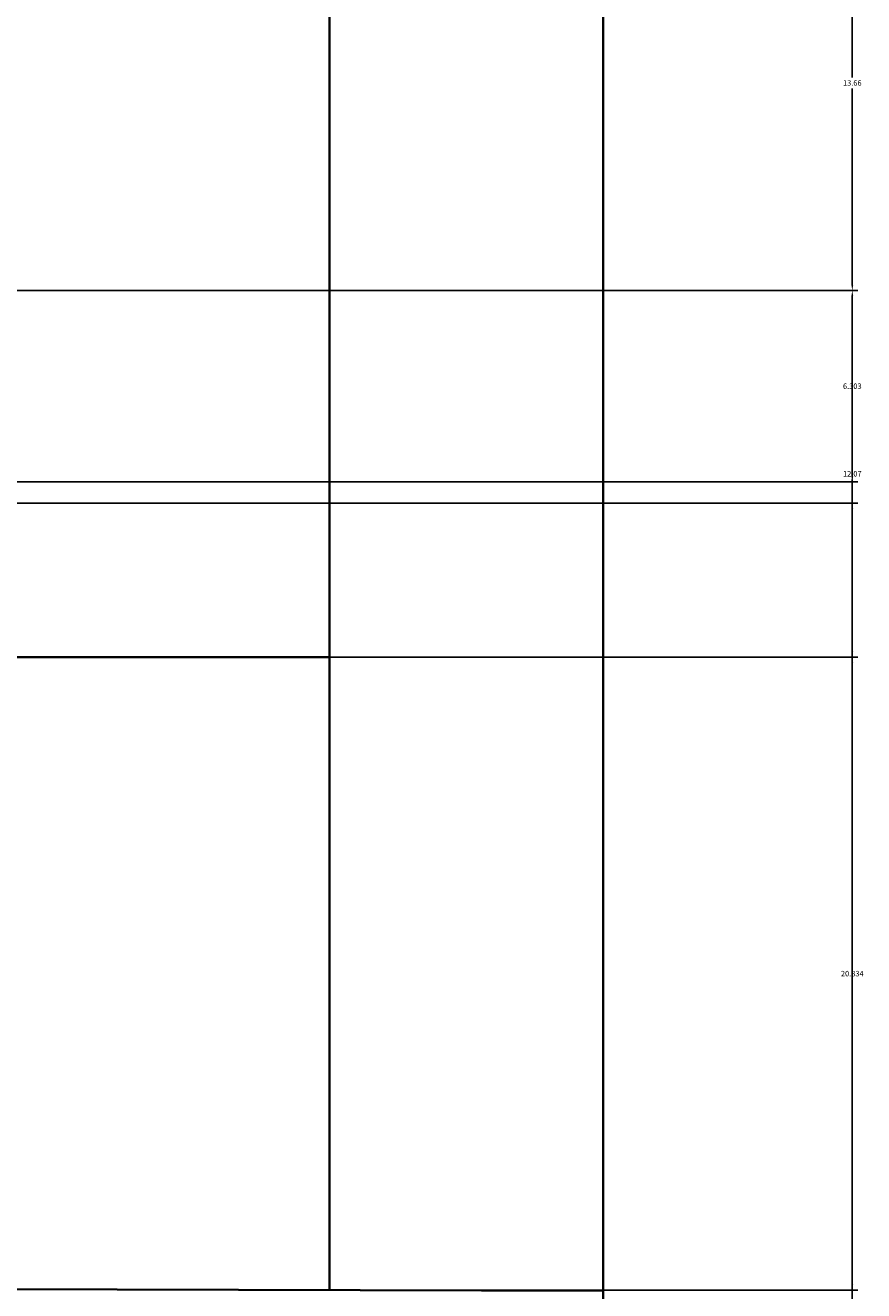
# Model space of a CAD drawing. Units: inches. Extents: x 27 to 200, y -50 to 102.
# Tile 23 of 26: x 172 to 200, y 19 to 61. Entities that reach past the tile are written whole.
import ezdxf

# ---------------------------------------------------------------- set-up
doc = ezdxf.new("R2010")
doc.units = ezdxf.units.IN
doc.header["$MEASUREMENT"] = 0
doc.layers.add('A-ANNO-DIMS', color=2, linetype='Continuous', lineweight=18)
doc.layers.add('A-ELEV', color=7, linetype='Continuous', lineweight=35)
doc.styles.get("Standard").update_dxf_attribs({"font": 'arial.ttf'})
doc.dimstyles.get("Standard").update_dxf_attribs({"dimtxt": 0.18, "dimasz": 0.18, "dimexe": 0.18, "dimexo": 0.0625, "dimgap": 0.09, "dimtad": 0, "dimtih": 1, "dimtoh": 1, "dimdec": 4, "dimzin": 0, "dimdsep": 46, "dimtxsty": 'Standard', "dimcen": 0.09, "dimadec": 0, "dimazin": 0, "dimtfac": 1, "dimtdec": 4, "dimtofl": 0, "dimtmove": 0, "dimatfit": 3, "dimfxl": 1, "dimtolj": 1, "dimtzin": 0, "dimarcsym": 0})

# ---------------------------------------------------------------- blocks, each defined once
blk = doc.blocks.new('*D27')
at = {"layer": 'A-ANNO-DIMS', "color": 0, "lineweight": -2, "transparency": 16777216}
for p, q in [((182.479, 39.856), (199.797, 39.856)), ((199.617, 39.676), (199.617, 29.621)), ((199.617, 19.202), (199.617, 29.257)), ((182.479, 19.022), (199.797, 19.022))]:
    blk.add_line(p, q, dxfattribs=at)
at = {"layer": 'A-ANNO-DIMS', "color": 0, "transparency": 16777216}
for points in [[(199.587, 39.676), (199.647, 39.676), (199.617, 39.856)], [(199.587, 19.202), (199.647, 19.202), (199.617, 19.022)]]:
    blk.add_solid(points, dxfattribs=at)
at = {"layer": 'Defpoints', "color": 0, "transparency": 16777216}
for p in [(182.417, 39.856), (199.617, 39.856), (182.417, 19.022)]:
    blk.add_point(p, dxfattribs=at)
at = {"layer": 'A-ANNO-DIMS', "color": 0, "transparency": 16777216, "insert": (199.617, 29.439), "char_height": 0.18, "attachment_point": 5}
blk.add_mtext('\\A1;20.834', dxfattribs=at)
blk = doc.blocks.new('*D28')
at = {"layer": 'A-ANNO-DIMS', "color": 0, "lineweight": -2, "transparency": 16777216}
for p, q in [((146.479, 51.926), (199.797, 51.926)), ((199.617, 51.746), (199.617, 46.073)), ((199.617, 40.036), (199.617, 45.709)), ((146.479, 39.856), (199.797, 39.856))]:
    blk.add_line(p, q, dxfattribs=at)
at = {"layer": 'A-ANNO-DIMS', "color": 0, "transparency": 16777216}
for points in [[(199.587, 51.746), (199.647, 51.746), (199.617, 51.926)], [(199.587, 40.036), (199.647, 40.036), (199.617, 39.856)]]:
    blk.add_solid(points, dxfattribs=at)
at = {"layer": 'Defpoints', "color": 0, "transparency": 16777216}
for p in [(146.417, 51.926), (199.617, 51.926), (146.417, 39.856)]:
    blk.add_point(p, dxfattribs=at)
at = {"layer": 'A-ANNO-DIMS', "color": 0, "transparency": 16777216, "insert": (199.617, 45.891), "char_height": 0.18, "attachment_point": 5}
blk.add_mtext('\\A1;12.07', dxfattribs=at)
blk = doc.blocks.new('*D29')
at = {"layer": 'A-ANNO-DIMS', "color": 0, "lineweight": -2, "transparency": 16777216}
for p, q in [((146.479, 65.587), (199.797, 65.587)), ((199.617, 65.407), (199.617, 58.938)), ((199.617, 52.106), (199.617, 58.575)), ((146.479, 51.926), (199.797, 51.926))]:
    blk.add_line(p, q, dxfattribs=at)
at = {"layer": 'A-ANNO-DIMS', "color": 0, "transparency": 16777216}
for points in [[(199.587, 65.407), (199.647, 65.407), (199.617, 65.587)], [(199.587, 52.106), (199.647, 52.106), (199.617, 51.926)]]:
    blk.add_solid(points, dxfattribs=at)
at = {"layer": 'Defpoints', "color": 0, "transparency": 16777216}
for p in [(146.417, 65.587), (199.617, 65.587), (146.417, 51.926)]:
    blk.add_point(p, dxfattribs=at)
at = {"layer": 'A-ANNO-DIMS', "color": 0, "transparency": 16777216, "insert": (199.617, 58.756), "char_height": 0.18, "attachment_point": 5}
blk.add_mtext('\\A1;13.66', dxfattribs=at)
blk = doc.blocks.new('*D48')
at = {"layer": 'A-ANNO-DIMS', "color": 0, "lineweight": -2, "transparency": 16777216}
for p, q in [((84.479, 44.926), (199.797, 44.926)), ((199.617, 44.746), (199.617, 14.26)), ((199.617, -16.589), (199.617, 13.897)), ((84.479, -16.769), (199.797, -16.769))]:
    blk.add_line(p, q, dxfattribs=at)
at = {"layer": 'A-ANNO-DIMS', "color": 0, "transparency": 16777216}
for points in [[(199.587, 44.746), (199.647, 44.746), (199.617, 44.926)], [(199.587, -16.589), (199.647, -16.589), (199.617, -16.769)]]:
    blk.add_solid(points, dxfattribs=at)
at = {"layer": 'Defpoints', "color": 0, "transparency": 16777216}
for p in [(84.417, 44.926), (199.617, 44.926), (84.417, -16.769)]:
    blk.add_point(p, dxfattribs=at)
at = {"layer": 'A-ANNO-DIMS', "color": 0, "transparency": 16777216, "insert": (199.617, 14.079), "char_height": 0.18, "attachment_point": 5}
blk.add_mtext('\\A1;61.7', dxfattribs=at)
blk = doc.blocks.new('*D52')
at = {"layer": 'A-ANNO-DIMS', "color": 0, "lineweight": -2, "transparency": 16777216}
for p, q in [((146.479, 51.926), (199.797, 51.926)), ((199.617, 51.746), (199.617, 48.957)), ((199.617, 45.803), (199.617, 48.593)), ((146.479, 45.623), (199.797, 45.623))]:
    blk.add_line(p, q, dxfattribs=at)
at = {"layer": 'A-ANNO-DIMS', "color": 0, "transparency": 16777216}
for points in [[(199.587, 51.746), (199.647, 51.746), (199.617, 51.926)], [(199.587, 45.803), (199.647, 45.803), (199.617, 45.623)]]:
    blk.add_solid(points, dxfattribs=at)
at = {"layer": 'Defpoints', "color": 0, "transparency": 16777216}
for p in [(146.417, 51.926), (199.617, 51.926), (146.417, 45.623)]:
    blk.add_point(p, dxfattribs=at)
at = {"layer": 'A-ANNO-DIMS', "color": 0, "transparency": 16777216, "insert": (199.617, 48.775), "char_height": 0.18, "attachment_point": 5}
blk.add_mtext('\\A1;6.303', dxfattribs=at)

msp = doc.modelspace()

# ---------------------------------------------------------------- linework, layer by layer
at = {"layer": 'A-ELEV'}
for p, q in [((191.4169, 93.9264), (191.4169, -16.7693)), ((182.4169, 65.5865), (182.4169, 19.0222)), ((182.4169, 39.8559), (146.4169, 39.8559)), ((191.4169, 19.002), (89.3118, 19.2307))]:
    msp.add_line(p, q, dxfattribs=at)

# ---------------------------------------------------------------- dimensions: what is measured, and where the dimension line sits
at = {"layer": 'A-ANNO-DIMS'}
for base, p1, p2, override, picture, middle in [((199.6169, 65.5865), (146.4169, 51.9264), (146.4169, 65.5865), {"dimdec": 2, "dimlfac": 1, "dimrnd": 0, "dimzin": 0, "dimdsep": 46, "dimlunit": 2}, '*D29', (199.6169, 58.7565)), ((199.6169, 51.9264), (146.4169, 39.8559), (146.4169, 51.9264), {"dimdec": 2, "dimlfac": 1, "dimrnd": 0, "dimzin": 0, "dimdsep": 46, "dimlunit": 2}, '*D28', (199.6169, 45.8912)), ((199.6169, 51.9264), (146.4169, 45.6231), (146.4169, 51.9264), {"dimdec": 3, "dimlfac": 1, "dimrnd": 0, "dimzin": 0, "dimdsep": 46, "dimlunit": 2}, '*D52', (199.6169, 48.7748)), ((199.6169, 44.9264), (84.4169, -16.7693), (84.4169, 44.9264), {"dimdec": 1, "dimlfac": 1, "dimrnd": 0, "dimzin": 0, "dimdsep": 46, "dimlunit": 2}, '*D48', (199.6169, 14.0786)), ((199.6169, 39.8559), (182.4169, 19.0222), (182.4169, 39.8559), {"dimdec": 3, "dimlfac": 1, "dimrnd": 0, "dimzin": 0, "dimdsep": 46, "dimlunit": 2}, '*D27', (199.6169, 29.439))]:
    dim = msp.add_linear_dim(base=base, p1=p1, p2=p2, angle=90, dimstyle='Standard', override=override, dxfattribs=at)
    dim.commit()
    dim.dimension.update_dxf_attribs({"geometry": picture, "text_midpoint": middle})

doc.saveas('drawing.dxf')
